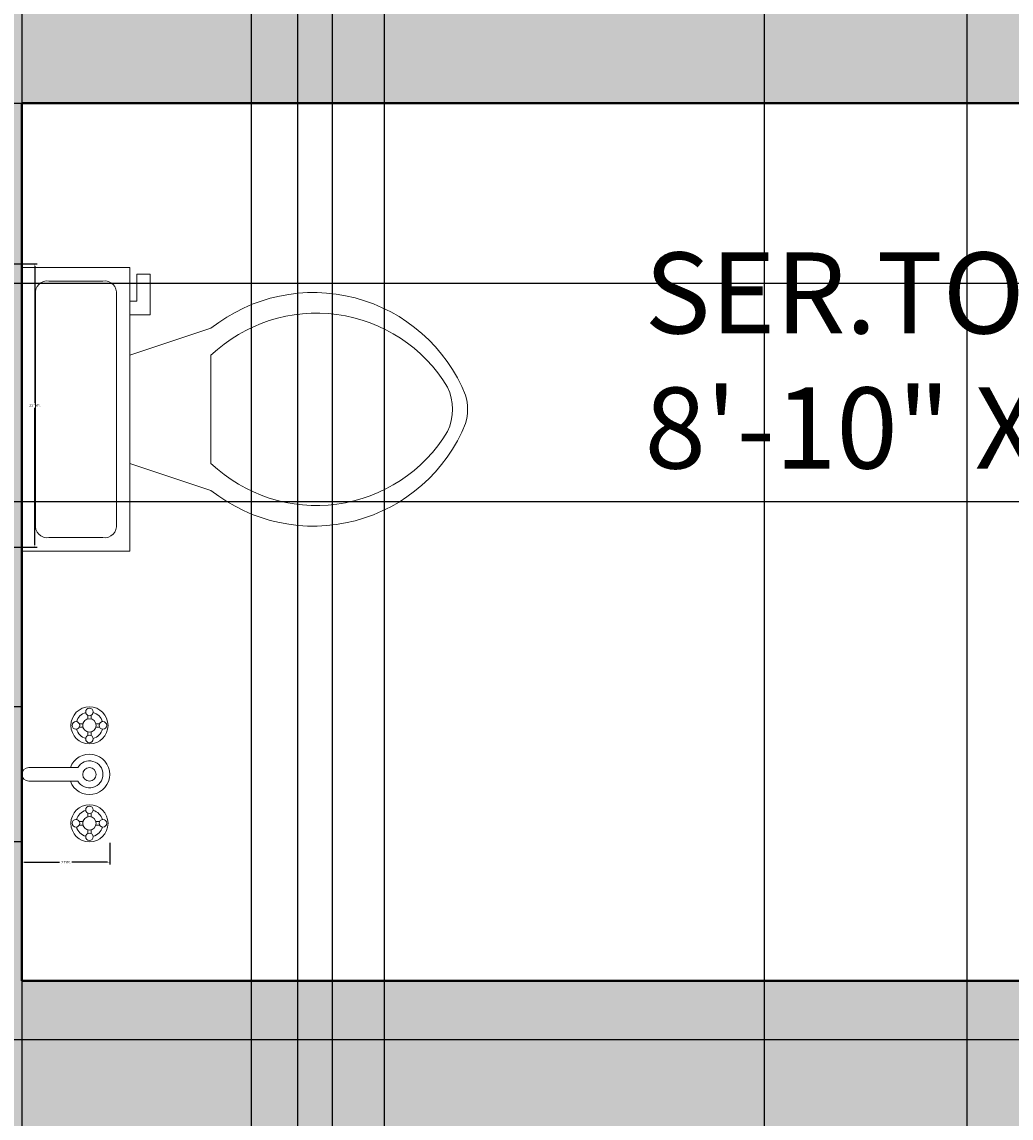
# Model space of a CAD drawing. Units: inches. Extents: x 818 to 1898, y 976 to 2364.
# Tile 54 of 96: x 1600 to 1673, y 1792 to 1873. Entities that reach past the tile are written whole.
import ezdxf

# ---------------------------------------------------------------- set-up
doc = ezdxf.new("R2010")
doc.units = ezdxf.units.IN
doc.header["$LTSCALE"] = 5
doc.header["$MEASUREMENT"] = 0
for name, color, linetype, lineweight in [('A-ANNO-DIMS', 2, 'Continuous', 18), ('A-AREA-IDEN', 7, 'Continuous', 18), ('A-FLOR-FIXT', 9, 'Continuous', 18), ('A-WALL', 7, 'Continuous', 40)]:
    doc.layers.add(name, color=color, linetype=linetype, lineweight=lineweight)
doc.layers.add('A-WALL-PATT', color=251, linetype='Continuous', lineweight=13, true_color=0x636466)
doc.styles.get("Standard").update_dxf_attribs({"font": 'arial.ttf'})
doc.dimstyles.get("Standard").update_dxf_attribs({"dimtxt": 0.18, "dimasz": 0.18, "dimexe": 0.18, "dimexo": 0.0625, "dimgap": 0.09, "dimtad": 0, "dimtih": 1, "dimtoh": 1, "dimdec": 4, "dimzin": 0, "dimdsep": 46, "dimtxsty": 'Standard', "dimcen": 0.09, "dimadec": 0, "dimazin": 0, "dimtfac": 1, "dimtdec": 4, "dimtofl": 0, "dimtmove": 0, "dimatfit": 3, "dimfxl": 1, "dimtolj": 1, "dimtzin": 0, "dimarcsym": 0})

# ---------------------------------------------------------------- blocks, each defined once
blk = doc.blocks.new('Toilet - top')
for p, q in [((9.5, -6), (9.5, -2)), ((-8, -8.5), (-8, -8)), ((-7, -8), (-7, -9.5)), ((-4, -8), (-6, -14)), ((4, -8), (6, -14)), ((-10, -8.5), (-8, -8.5)), ((-10, -9.5), (-10, -8.5)), ((-7, -9.5), (-10, -9.5)), ((4, -14), (-4, -14))]:
    blk.add_line(p, q)
blk.add_lwpolyline([(10.5, -8), (10.5, 0), (-10.5, 0), (-10.5, -8)], close=True)
for points in [[(8.5, -1), (-8.5, -1)], [(-9.5, -2), (-9.5, -6)], [(-8.5, -7), (8.5, -7)]]:
    blk.add_lwpolyline(points)
for centre, radius, start, end in [((-8.625, -1.875), 0.884, 81.8699, 188.1301), ((8.625, -1.875), 0.884, 351.8699, 98.1301), ((-8.625, -6.125), 0.884, 171.8699, 278.1301), ((8.625, -6.125), 0.884, 261.8699, 8.1301), ((3.52, -21.58), 12.169, 141.46911, 247.97143), ((4.2, -21.817), 11.329, 136.36773, 238.94682), ((-3.519, -21.58), 12.169, 292.02843, 38.53071), ((-4.2, -21.817), 11.329, 301.05301, 43.63209), ((0, -27.876), 4, 245.73182, 294.26817), ((0, -29), 4, 254.86053, 285.13947)]:
    blk.add_arc(centre, radius, start, end)
blk = doc.blocks.new('Faucet - Bathroom top')
for p, q in [((-4.107, 0.125), (-4.375, 0.125)), ((-3.75, 0.4788), (-3.75, 0.75)), ((-3.5, 0.482), (-3.5, 0.75)), ((-3.1461, 0.125), (-2.875, 0.125)), ((3.143, 0.125), (2.875, 0.125)), ((3.5, 0.4788), (3.5, 0.75)), ((3.75, 0.482), (3.75, 0.75)), ((4.1039, 0.125), (4.375, 0.125)), ((-4.1039, -0.125), (-4.375, -0.125)), ((-3.75, -0.4821), (-3.75, -0.75)), ((-3.5, -0.4789), (-3.5, -0.75)), ((-3.143, -0.125), (-2.875, -0.125)), ((3.1461, -0.125), (2.875, -0.125)), ((3.5, -0.4821), (3.5, -0.75)), ((3.75, -0.4789), (3.75, -0.75)), ((4.107, -0.125), (4.375, -0.125)), ((-0.5, -0.8639), (-0.5, -4.5)), ((0.5, -4.5), (0.5, -0.8631))]:
    blk.add_line(p, q)
for centre, radius in [((-3.625, 0), 1.375), ((-3.625, 1), 0.2795), ((3.625, 0), 1.375), ((3.625, 1), 0.2795), ((-4.625, 0), 0.2795), ((-3.625, 0), 0.5), ((-2.625, 0), 0.2795), ((0, 0), 0.5), ((2.625, 0), 0.2795), ((3.625, 0), 0.5), ((4.625, 0), 0.2795), ((-3.625, -1), 0.2795), ((3.625, -1), 0.2795)]:
    blk.add_circle(centre, radius)
for centre, radius, start, end in [((-3.625, 0), 1, 105.2407, 164.2093), ((-3.625, 0), 1, 16.44125, 74.07887), ((0, 0), 1.5, 289.6514, 250.3603), ((0, 0), 1, 300.3431, 239.7554), ((3.625, 0), 1, 106.12, 164.0884), ((3.625, 0), 1, 16.23422, 73.90469), ((-3.625, 0), 1, 196.2342, 253.9047), ((-3.625, 0), 1, 286.12, 344.0884), ((3.625, 0), 1, 196.4413, 254.0789), ((3.625, 0), 1, 285.2407, 344.2093), ((0, -4.5), 0.5, 180, 0)]:
    blk.add_arc(centre, radius, start, end)
blk = doc.blocks.new('*D36')
at = {"layer": 'A-ANNO-DIMS', "color": 0, "lineweight": -2, "ltscale": 5, "transparency": 16777216}
for p, q in [((1599.663, 1822.366), (1598.045, 1822.366)), ((1598.225, 1822.186), (1598.225, 1817.548)), ((1598.225, 1812.546), (1598.225, 1817.184)), ((1599.663, 1812.366), (1598.045, 1812.366))]:
    blk.add_line(p, q, dxfattribs=at)
at = {"layer": 'A-ANNO-DIMS', "color": 0, "ltscale": 5, "transparency": 16777216}
for points in [[(1598.195, 1822.186), (1598.255, 1822.186), (1598.225, 1822.366)], [(1598.195, 1812.546), (1598.255, 1812.546), (1598.225, 1812.366)]]:
    blk.add_solid(points, dxfattribs=at)
at = {"layer": 'Defpoints', "color": 0, "ltscale": 5, "transparency": 16777216}
for p in [(1599.725, 1822.366), (1598.225, 1812.366), (1599.725, 1812.366)]:
    blk.add_point(p, dxfattribs=at)
at = {"layer": 'A-ANNO-DIMS', "color": 0, "ltscale": 5, "transparency": 16777216, "insert": (1598.225, 1817.366), "char_height": 0.18, "attachment_point": 5}
blk.add_mtext('\\A1;TAP 10 TYP.', dxfattribs=at)
blk = doc.blocks.new('*D37')
at = {"layer": 'A-ANNO-DIMS', "color": 0, "lineweight": -2, "ltscale": 5, "transparency": 16777216}
for p, q in [((1599.725, 1812.304), (1599.725, 1810.686)), ((1606.225, 1812.304), (1606.225, 1810.686)), ((1599.905, 1810.866), (1602.518, 1810.866)), ((1606.045, 1810.866), (1603.433, 1810.866))]:
    blk.add_line(p, q, dxfattribs=at)
at = {"layer": 'A-ANNO-DIMS', "color": 0, "ltscale": 5, "transparency": 16777216}
for points in [[(1599.905, 1810.896), (1599.905, 1810.836), (1599.725, 1810.866)], [(1606.045, 1810.896), (1606.045, 1810.836), (1606.225, 1810.866)]]:
    blk.add_solid(points, dxfattribs=at)
at = {"layer": 'Defpoints', "color": 0, "ltscale": 5, "transparency": 16777216}
for p in [(1599.725, 1812.366), (1606.225, 1812.366), (1606.225, 1810.866)]:
    blk.add_point(p, dxfattribs=at)
at = {"layer": 'A-ANNO-DIMS', "color": 0, "ltscale": 5, "transparency": 16777216, "insert": (1602.975, 1810.866), "char_height": 0.18, "attachment_point": 5}
blk.add_mtext('\\A1;7 TYP.', dxfattribs=at)
blk = doc.blocks.new('*D41')
at = {"layer": 'A-ANNO-DIMS', "color": 0, "lineweight": -2, "ltscale": 5, "transparency": 16777216}
for p, q in [((1595.788, 1855.184), (1600.862, 1855.184)), ((1600.682, 1855.004), (1600.682, 1844.865)), ((1600.682, 1834.364), (1600.682, 1844.504)), ((1595.788, 1834.184), (1600.862, 1834.184))]:
    blk.add_line(p, q, dxfattribs=at)
at = {"layer": 'A-ANNO-DIMS', "color": 0, "ltscale": 5, "transparency": 16777216}
for points in [[(1600.652, 1855.004), (1600.712, 1855.004), (1600.682, 1855.184)], [(1600.652, 1834.364), (1600.712, 1834.364), (1600.682, 1834.184)]]:
    blk.add_solid(points, dxfattribs=at)
at = {"layer": 'Defpoints', "color": 0, "ltscale": 5, "transparency": 16777216}
for p in [(1595.725, 1855.184), (1595.725, 1834.184), (1600.682, 1834.184)]:
    blk.add_point(p, dxfattribs=at)
at = {"layer": 'A-ANNO-DIMS', "color": 0, "ltscale": 5, "transparency": 16777216, "insert": (1600.682, 1844.684), "char_height": 0.18, "attachment_point": 5}
blk.add_mtext('\\A1;21 TYP.', dxfattribs=at)
blk = doc.blocks.new('*D85')
at = {"layer": 'A-ANNO-DIMS', "color": 0, "lineweight": -2, "ltscale": 5, "transparency": 16777216}
for p, q in [((1258.788, 2053.078), (1897.916, 2053.078)), ((1897.736, 2052.898), (1897.736, 1876.76)), ((1897.736, 1700.258), (1897.736, 1876.396)), ((1258.788, 1700.078), (1897.916, 1700.078))]:
    blk.add_line(p, q, dxfattribs=at)
at = {"layer": 'A-ANNO-DIMS', "color": 0, "ltscale": 5, "transparency": 16777216}
for points in [[(1897.706, 2052.898), (1897.766, 2052.898), (1897.736, 2053.078)], [(1897.706, 1700.258), (1897.766, 1700.258), (1897.736, 1700.078)]]:
    blk.add_solid(points, dxfattribs=at)
at = {"layer": 'Defpoints', "color": 0, "ltscale": 5, "transparency": 16777216}
for p in [(1258.725, 2053.078), (1897.736, 2053.078), (1258.725, 1700.078)]:
    blk.add_point(p, dxfattribs=at)
at = {"layer": 'A-ANNO-DIMS', "color": 0, "ltscale": 5, "transparency": 16777216, "insert": (1897.736, 1876.578), "char_height": 0.18, "attachment_point": 5}
blk.add_mtext('\\A1;353', dxfattribs=at)
blk = doc.blocks.new('*D102')
at = {"layer": 'A-ANNO-DIMS', "color": 0, "lineweight": -2, "ltscale": 5, "transparency": 16777216}
for p, q in [((1565.483, 1071.118), (1565.483, 2363.873)), ((1565.663, 2363.693), (1595.635, 2363.693)), ((1626.395, 2363.693), (1596.423, 2363.693)), ((1626.575, 1071.118), (1626.575, 2363.873))]:
    blk.add_line(p, q, dxfattribs=at)
at = {"layer": 'A-ANNO-DIMS', "color": 0, "ltscale": 5, "transparency": 16777216}
for points in [[(1565.663, 2363.723), (1565.663, 2363.663), (1565.483, 2363.693)], [(1626.395, 2363.723), (1626.395, 2363.663), (1626.575, 2363.693)]]:
    blk.add_solid(points, dxfattribs=at)
at = {"layer": 'Defpoints', "color": 0, "ltscale": 5, "transparency": 16777216}
for p in [(1626.575, 2363.693), (1565.483, 1071.055), (1626.575, 1071.055)]:
    blk.add_point(p, dxfattribs=at)
at = {"layer": 'A-ANNO-DIMS', "color": 0, "ltscale": 5, "transparency": 16777216, "insert": (1596.029, 2363.693), "char_height": 0.18, "attachment_point": 5}
blk.add_mtext('\\A1;61.09', dxfattribs=at)
blk = doc.blocks.new('*D103')
at = {"layer": 'A-ANNO-DIMS', "color": 0, "lineweight": -2, "ltscale": 5, "transparency": 16777216}
for p, q in [((1626.575, 1071.118), (1626.575, 2363.873)), ((1626.755, 2363.693), (1657.699, 2363.693)), ((1689.291, 2363.693), (1658.348, 2363.693)), ((1689.471, 1071.118), (1689.471, 2363.873))]:
    blk.add_line(p, q, dxfattribs=at)
at = {"layer": 'A-ANNO-DIMS', "color": 0, "ltscale": 5, "transparency": 16777216}
for points in [[(1626.755, 2363.723), (1626.755, 2363.663), (1626.575, 2363.693)], [(1689.291, 2363.723), (1689.291, 2363.663), (1689.471, 2363.693)]]:
    blk.add_solid(points, dxfattribs=at)
at = {"layer": 'Defpoints', "color": 0, "ltscale": 5, "transparency": 16777216}
for p in [(1689.471, 2363.693), (1626.575, 1071.055), (1689.471, 1071.055)]:
    blk.add_point(p, dxfattribs=at)
at = {"layer": 'A-ANNO-DIMS', "color": 0, "ltscale": 5, "transparency": 16777216, "insert": (1658.023, 2363.693), "char_height": 0.18, "attachment_point": 5}
blk.add_mtext('\\A1;62.9', dxfattribs=at)
blk = doc.blocks.new('*D120')
at = {"layer": 'A-ANNO-DIMS', "color": 0, "lineweight": -2, "ltscale": 5, "transparency": 16777216}
for p, q in [((1766.29, 1797.717), (818.026, 1797.717)), ((818.206, 1797.537), (818.206, 1757.534)), ((818.206, 1717.167), (818.206, 1757.17)), ((1766.29, 1716.987), (818.026, 1716.987))]:
    blk.add_line(p, q, dxfattribs=at)
at = {"layer": 'A-ANNO-DIMS', "color": 0, "ltscale": 5, "transparency": 16777216}
for points in [[(818.176, 1797.537), (818.236, 1797.537), (818.206, 1797.717)], [(818.176, 1717.167), (818.236, 1717.167), (818.206, 1716.987)]]:
    blk.add_solid(points, dxfattribs=at)
at = {"layer": 'Defpoints', "color": 0, "ltscale": 5, "transparency": 16777216}
for p in [(818.206, 1797.717), (1766.352, 1797.717), (1766.352, 1716.987)]:
    blk.add_point(p, dxfattribs=at)
at = {"layer": 'A-ANNO-DIMS', "color": 0, "ltscale": 5, "transparency": 16777216, "insert": (818.206, 1757.352), "char_height": 0.18, "attachment_point": 5}
blk.add_mtext('\\A1;80.73', dxfattribs=at)
blk = doc.blocks.new('*D121')
at = {"layer": 'A-ANNO-DIMS', "color": 0, "lineweight": -2, "ltscale": 5, "transparency": 16777216}
for p, q in [((1766.29, 1884.203), (818.026, 1884.203)), ((818.206, 1884.023), (818.206, 1841.142)), ((818.206, 1797.897), (818.206, 1840.778)), ((1766.29, 1797.717), (818.026, 1797.717))]:
    blk.add_line(p, q, dxfattribs=at)
at = {"layer": 'A-ANNO-DIMS', "color": 0, "ltscale": 5, "transparency": 16777216}
for points in [[(818.176, 1884.023), (818.236, 1884.023), (818.206, 1884.203)], [(818.176, 1797.897), (818.236, 1797.897), (818.206, 1797.717)]]:
    blk.add_solid(points, dxfattribs=at)
at = {"layer": 'Defpoints', "color": 0, "ltscale": 5, "transparency": 16777216}
for p in [(818.206, 1884.203), (1766.352, 1884.203), (1766.352, 1797.717)]:
    blk.add_point(p, dxfattribs=at)
at = {"layer": 'A-ANNO-DIMS', "color": 0, "ltscale": 5, "transparency": 16777216, "insert": (818.206, 1840.96), "char_height": 0.18, "attachment_point": 5}
blk.add_mtext('\\A1;86.49', dxfattribs=at)
blk = doc.blocks.new('*D173')
at = {"layer": 'A-ANNO-DIMS', "color": 0, "lineweight": -2, "ltscale": 5, "transparency": 16777216}
for p, q in [((1622.725, 1463.141), (1622.725, 2363.873)), ((1622.905, 2363.693), (1638.507, 2363.693)), ((1654.545, 2363.693), (1638.943, 2363.693)), ((1654.725, 1463.141), (1654.725, 2363.873))]:
    blk.add_line(p, q, dxfattribs=at)
at = {"layer": 'A-ANNO-DIMS', "color": 0, "ltscale": 5, "transparency": 16777216}
for points in [[(1622.905, 2363.723), (1622.905, 2363.663), (1622.725, 2363.693)], [(1654.545, 2363.723), (1654.545, 2363.663), (1654.725, 2363.693)]]:
    blk.add_solid(points, dxfattribs=at)
at = {"layer": 'Defpoints', "color": 0, "ltscale": 5, "transparency": 16777216}
for p in [(1654.725, 2363.693), (1622.725, 1463.078), (1654.725, 1463.078)]:
    blk.add_point(p, dxfattribs=at)
at = {"layer": 'A-ANNO-DIMS', "color": 0, "ltscale": 5, "transparency": 16777216, "insert": (1638.725, 2363.693), "char_height": 0.18, "attachment_point": 5}
blk.add_mtext('\\A1;32', dxfattribs=at)
blk = doc.blocks.new('*D174')
at = {"layer": 'A-ANNO-DIMS', "color": 0, "lineweight": -2, "ltscale": 5, "transparency": 16777216}
for p, q in [((1616.725, 1416.748), (1616.725, 2363.873)), ((1616.905, 2363.693), (1619.576, 2363.693)), ((1622.545, 2363.693), (1619.875, 2363.693)), ((1622.725, 1416.748), (1622.725, 2363.873))]:
    blk.add_line(p, q, dxfattribs=at)
at = {"layer": 'A-ANNO-DIMS', "color": 0, "ltscale": 5, "transparency": 16777216}
for points in [[(1616.905, 2363.723), (1616.905, 2363.663), (1616.725, 2363.693)], [(1622.545, 2363.723), (1622.545, 2363.663), (1622.725, 2363.693)]]:
    blk.add_solid(points, dxfattribs=at)
at = {"layer": 'Defpoints', "color": 0, "ltscale": 5, "transparency": 16777216}
for p in [(1622.725, 2363.693), (1616.725, 1416.686), (1622.725, 1416.686)]:
    blk.add_point(p, dxfattribs=at)
at = {"layer": 'A-ANNO-DIMS', "color": 0, "ltscale": 5, "transparency": 16777216, "insert": (1619.725, 2363.693), "char_height": 0.18, "attachment_point": 5}
blk.add_mtext('\\A1;6', dxfattribs=at)
blk = doc.blocks.new('*D175')
at = {"layer": 'A-ANNO-DIMS', "color": 0, "lineweight": -2, "ltscale": 5, "transparency": 16777216}
for p, q in [((1559.725, 1647.641), (1559.725, 2363.873)), ((1559.905, 2363.693), (1614.445, 2363.693)), ((1669.545, 2363.693), (1615.005, 2363.693)), ((1669.725, 1647.641), (1669.725, 2363.873))]:
    blk.add_line(p, q, dxfattribs=at)
at = {"layer": 'A-ANNO-DIMS', "color": 0, "ltscale": 5, "transparency": 16777216}
for points in [[(1559.905, 2363.723), (1559.905, 2363.663), (1559.725, 2363.693)], [(1669.545, 2363.723), (1669.545, 2363.663), (1669.725, 2363.693)]]:
    blk.add_solid(points, dxfattribs=at)
at = {"layer": 'Defpoints', "color": 0, "ltscale": 5, "transparency": 16777216}
for p in [(1669.725, 2363.693), (1559.725, 1647.578), (1669.725, 1647.578)]:
    blk.add_point(p, dxfattribs=at)
at = {"layer": 'A-ANNO-DIMS', "color": 0, "ltscale": 5, "transparency": 16777216, "insert": (1614.725, 2363.693), "char_height": 0.18, "attachment_point": 5}
blk.add_mtext('\\A1;110', dxfattribs=at)
blk = doc.blocks.new('*D225')
at = {"layer": 'A-ANNO-DIMS', "color": 0, "lineweight": -2, "ltscale": 5, "transparency": 16777216}
for p, q in [((1532.655, 1867.078), (1897.916, 1867.078)), ((1897.736, 1866.898), (1897.736, 1852.512)), ((1897.736, 1837.762), (1897.736, 1852.148)), ((1532.655, 1837.582), (1897.916, 1837.582))]:
    blk.add_line(p, q, dxfattribs=at)
at = {"layer": 'A-ANNO-DIMS', "color": 0, "ltscale": 5, "transparency": 16777216}
for points in [[(1897.706, 1866.898), (1897.766, 1866.898), (1897.736, 1867.078)], [(1897.706, 1837.762), (1897.766, 1837.762), (1897.736, 1837.582)]]:
    blk.add_solid(points, dxfattribs=at)
at = {"layer": 'Defpoints', "color": 0, "ltscale": 5, "transparency": 16777216}
for p in [(1532.593, 1867.078), (1897.736, 1867.078), (1532.593, 1837.582)]:
    blk.add_point(p, dxfattribs=at)
at = {"layer": 'A-ANNO-DIMS', "color": 0, "ltscale": 5, "transparency": 16777216, "insert": (1897.736, 1852.33), "char_height": 0.18, "attachment_point": 5}
blk.add_mtext('\\A1;29.496', dxfattribs=at)
blk = doc.blocks.new('*D229')
at = {"layer": 'A-ANNO-DIMS', "color": 0, "lineweight": -2, "ltscale": 5, "transparency": 16777216}
for p, q in [((1599.725, 2044.016), (1599.725, 975.663)), ((1620.142, 2036.056), (1620.142, 975.663)), ((1599.905, 975.843), (1609.468, 975.843)), ((1619.962, 975.843), (1610.398, 975.843))]:
    blk.add_line(p, q, dxfattribs=at)
at = {"layer": 'A-ANNO-DIMS', "color": 0, "ltscale": 5, "transparency": 16777216}
for points in [[(1599.905, 975.873), (1599.905, 975.813), (1599.725, 975.843)], [(1619.962, 975.873), (1619.962, 975.813), (1620.142, 975.843)]]:
    blk.add_solid(points, dxfattribs=at)
at = {"layer": 'Defpoints', "color": 0, "ltscale": 5, "transparency": 16777216}
for p in [(1599.725, 2044.078), (1620.142, 2036.118), (1620.142, 975.843)]:
    blk.add_point(p, dxfattribs=at)
at = {"layer": 'A-ANNO-DIMS', "color": 0, "ltscale": 5, "transparency": 16777216, "insert": (1609.933, 975.843), "char_height": 0.18, "attachment_point": 5}
blk.add_mtext('\\A1;20.416', dxfattribs=at)
blk = doc.blocks.new('*D275')
at = {"layer": 'A-ANNO-DIMS', "color": 0, "lineweight": -2, "ltscale": 5, "transparency": 16777216}
for p, q in [((1377.842, 1897.866), (1897.916, 1897.866)), ((1897.736, 1897.686), (1897.736, 1875.988)), ((1897.736, 1853.93), (1897.736, 1875.628)), ((1377.842, 1853.75), (1897.916, 1853.75))]:
    blk.add_line(p, q, dxfattribs=at)
at = {"layer": 'A-ANNO-DIMS', "color": 0, "ltscale": 5, "transparency": 16777216}
for points in [[(1897.706, 1897.686), (1897.766, 1897.686), (1897.736, 1897.866)], [(1897.706, 1853.93), (1897.766, 1853.93), (1897.736, 1853.75)]]:
    blk.add_solid(points, dxfattribs=at)
at = {"layer": 'Defpoints', "color": 0, "ltscale": 5, "transparency": 16777216}
for p in [(1377.779, 1897.866), (1897.736, 1897.866), (1377.779, 1853.75)]:
    blk.add_point(p, dxfattribs=at)
at = {"layer": 'A-ANNO-DIMS', "color": 0, "ltscale": 5, "transparency": 16777216, "insert": (1897.736, 1875.808), "char_height": 0.18, "attachment_point": 5}
blk.add_mtext('\\A1;44.12', dxfattribs=at)
blk = doc.blocks.new('*D282')
at = {"layer": 'A-ANNO-DIMS', "color": 0, "lineweight": -2, "ltscale": 5, "transparency": 16777216}
for p, q in [((1422.083, 2081.188), (1897.916, 2081.188)), ((1897.736, 2081.008), (1897.736, 1884.315)), ((1897.736, 1687.258), (1897.736, 1883.951)), ((1463.788, 1687.078), (1897.916, 1687.078))]:
    blk.add_line(p, q, dxfattribs=at)
at = {"layer": 'A-ANNO-DIMS', "color": 0, "ltscale": 5, "transparency": 16777216}
for points in [[(1897.706, 2081.008), (1897.766, 2081.008), (1897.736, 2081.188)], [(1897.706, 1687.258), (1897.766, 1687.258), (1897.736, 1687.078)]]:
    blk.add_solid(points, dxfattribs=at)
at = {"layer": 'Defpoints', "color": 0, "ltscale": 5, "transparency": 16777216}
for p in [(1422.02, 2081.188), (1897.736, 2081.188), (1463.725, 1687.078)]:
    blk.add_point(p, dxfattribs=at)
at = {"layer": 'A-ANNO-DIMS', "color": 0, "ltscale": 5, "transparency": 16777216, "insert": (1897.736, 1884.133), "char_height": 0.18, "attachment_point": 5}
blk.add_mtext('\\A1;394.1', dxfattribs=at)

msp = doc.modelspace()

# ---------------------------------------------------------------- hatches: boundary and pattern name
at = {"layer": 'A-WALL-PATT', "ltscale": 5}
h = msp.add_hatch(color=256, dxfattribs=at)
h.dxf.hatch_style = 1
h.paths.add_polyline_path([(1267.7252, 1928.9218), (1258.7251, 1928.9218), (1258.7251, 1913.6401), (1250.3029, 1913.6401), (1250.3029, 1878.3919), (1258.7251, 1878.3919), (1258.7251, 1862.9652), (1267.7252, 1862.9652)])
h.paths.add_polyline_path([(1267.7252, 1814.9652), (1258.7251, 1814.9652), (1258.7251, 1755.3321), (1267.7252, 1755.3321)])
h.paths.add_polyline_path([(1463.7251, 1696.0782), (1267.7252, 1696.0782), (1267.7252, 1707.3321), (1258.7251, 1707.3321), (1258.7251, 1700.0782), (1251.9333, 1700.0782), (1251.9333, 1687.0782), (1463.7251, 1687.0782)])
h.paths.add_polyline_path([(1714.7252, 1717.3178), (1705.7252, 1717.3178), (1705.7252, 1696.0782), (1599.7251, 1696.0782), (1599.7251, 1790.0782), (1705.7252, 1790.0782), (1705.7252, 1785.6125), (1714.7252, 1785.6125), (1714.7252, 1827.2125), (1705.7252, 1827.2125), (1705.7252, 1802.0782), (1599.7251, 1802.0782), (1599.7251, 1867.0782), (1705.7252, 1867.0782), (1705.7252, 1857.2125), (1714.7252, 1857.2125), (1714.7252, 1930.0316), (1741.8409, 1930.0316), (1741.8409, 1935.0316), (1714.7252, 1935.0316), (1714.7252, 1957.0338), (1741.8409, 1957.0338), (1741.8409, 1962.0338), (1714.7252, 1962.0338), (1705.7252, 1962.0338), (1705.7252, 1948.0782), (1599.7251, 1948.0782), (1599.7251, 1981.0782), (1590.7252, 1981.0782), (1590.7252, 1941.0782), (1620.7252, 1941.0782), (1705.7252, 1941.0782), (1705.7252, 1876.0782), (1599.7251, 1876.0782), (1599.7251, 1911.0782), (1590.7252, 1911.0782), (1590.7252, 1876.0782), (1429.2252, 1876.0782), (1429.2252, 1867.0782), (1511.7252, 1867.0782), (1528.593, 1867.0782), (1595.7252, 1867.0782), (1595.7252, 1773.0782), (1520.7252, 1773.0782), (1520.7252, 1837.5823), (1532.593, 1837.5823), (1532.593, 1867.0782), (1528.593, 1867.0782), (1528.593, 1841.5823), (1511.7252, 1841.5823), (1511.7252, 1744.9714), (1520.7252, 1744.9714), (1520.7252, 1761.0782), (1595.7252, 1761.0782), (1595.7252, 1696.0782), (1520.7252, 1696.0782), (1520.7252, 1716.0454), (1511.7252, 1716.0454), (1511.7252, 1696.0782), (1511.7252, 1687.0782), (1714.7252, 1687.0782)])
h.paths.add_polyline_path([(1714.7252, 2053.0782), (1714.7252, 2081.1881), (1709.7252, 2081.1881), (1709.7252, 2053.0782), (1681.6446, 2053.0782), (1681.6446, 2081.1881), (1676.6446, 2081.1881), (1676.6446, 2053.0782), (1538.5155, 2053.0782), (1538.5155, 2044.0782), (1590.7252, 2044.0782), (1590.7252, 2011.0782), (1599.7251, 2011.0782), (1599.7251, 2044.0782), (1705.7252, 2044.0782), (1705.7252, 2014.5114), (1714.7252, 2014.5114)])
h.paths.add_polyline_path([(1485.1216, 2053.0782), (1422.02, 2053.0782), (1422.02, 2081.1881), (1413.02, 2081.1881), (1413.02, 2053.0782), (1399.6356, 2053.0782), (1399.6356, 2081.1881), (1390.6356, 2081.1881), (1390.6356, 2053.0782), (1388.0315, 2053.0782), (1388.0315, 2044.0782), (1416.2743, 2044.0782), (1485.1216, 2044.0782)])
h.paths.add_polyline_path([(1330.305, 2053.0782), (1258.7251, 2053.0782), (1258.7251, 2019.2871), (1267.7252, 2019.2871), (1267.7252, 2044.0782), (1330.305, 2044.0782)])
h.paths.add_polyline_path([(1258.7251, 2053.0782), (1214.6577, 2053.0782), (1214.6577, 2044.0782), (1258.7251, 2044.0782)])
h.paths.add_polyline_path([(1214.6577, 2053.0782), (1180.349, 2053.0782), (1180.349, 2044.0782), (1214.6577, 2044.0782)])
h.paths.add_polyline_path([(1714.7252, 1639.5782), (1741.8409, 1639.5782), (1741.8409, 1643.5782), (1714.7252, 1643.5782), (1714.7252, 1649.9029), (1705.7252, 1649.9029), (1705.7252, 1600.0782), (1477.7252, 1600.0782), (1477.7252, 1591.0782), (1520.7252, 1591.0782), (1616.7251, 1591.0782), (1616.7251, 1416.6857), (1622.7251, 1416.6857), (1622.7251, 1463.0782), (1624.7252, 1463.0782), (1624.7252, 1467.0782), (1622.7251, 1467.0782), (1622.7251, 1591.0782), (1705.7252, 1591.0782), (1705.7252, 1545.0782), (1714.7252, 1545.0782), (1741.8409, 1545.0782), (1741.8409, 1549.0782), (1714.7252, 1549.0782), (1714.7252, 1593.9175), (1737.8409, 1593.9175), (1737.8409, 1597.9175), (1714.7252, 1597.9175)])
h.paths.add_polyline_path([(1674.9024, 2060.7419), (1714.7045, 2060.7419), (1714.7045, 2073.1061), (1674.9024, 2073.1061)], flags=25)
h.paths.add_polyline_path([(1394.5468, 2061.6618), (1422.2344, 2061.6618), (1422.2344, 2074.0261), (1394.5468, 2074.0261)], flags=24)

# ---------------------------------------------------------------- linework, layer by layer
at = {"layer": 'A-WALL'}
for p, q in [((1599.7251, 1867.0782), (1705.7252, 1867.0782)), ((1599.7251, 1867.0782), (1599.7251, 1802.0782)), ((1599.7251, 1802.0782), (1705.7252, 1802.0782))]:
    msp.add_line(p, q, dxfattribs=at)

# ---------------------------------------------------------------- block references
at = {"layer": 'A-FLOR-FIXT', "xscale": -1, "rotation": 90}
msp.add_blockref('Toilet - top', (1599.7251, 1844.4024), dxfattribs=at)
at = {"layer": 'A-FLOR-FIXT', "rotation": 270}
msp.add_blockref('Faucet - Bathroom top', (1604.7252, 1817.3662), dxfattribs=at)

# ---------------------------------------------------------------- texts
at = {"layer": 'A-AREA-IDEN', "ltscale": 5, "insert": (1645.8362, 1856.0216), "char_height": 6, "attachment_point": 1}
msp.add_mtext_dynamic_manual_height_columns('SER.TOILET\\P8\'-10" X 5\'-5"', width=118.992422, gutter_width=1, heights=[0], dxfattribs=at)

# ---------------------------------------------------------------- dimensions: what is measured, and where the dimension line sits
at = {"layer": 'A-ANNO-DIMS', "ltscale": 5}
for base, p1, p2, override, picture, middle in [((1669.7251, 2363.6929), (1559.7251, 1647.5782), (1669.7251, 1647.5782), {"dimdec": 0, "dimlfac": 1, "dimrnd": 0, "dimzin": 0, "dimdsep": 46, "dimlunit": 2}, '*D175', (1614.7251, 2363.6929)), ((1626.5748, 2363.6929), (1565.4835, 1071.0552), (1626.5748, 1071.0552), {"dimdec": 2, "dimlfac": 1, "dimrnd": 0, "dimzin": 0, "dimdsep": 46, "dimlunit": 2}, '*D102', (1596.0291, 2363.6929)), ((1622.7251, 2363.6929), (1616.7251, 1416.6857), (1622.7251, 1416.6857), {"dimdec": 0, "dimlfac": 1, "dimrnd": 0, "dimzin": 0, "dimdsep": 46, "dimlunit": 2}, '*D174', (1619.7251, 2363.6929)), ((1654.7251, 2363.6929), (1622.7251, 1463.0782), (1654.7251, 1463.0782), {"dimdec": 0, "dimlfac": 1, "dimrnd": 0, "dimzin": 0, "dimdsep": 46, "dimlunit": 2}, '*D173', (1638.7251, 2363.6929)), ((1689.4714, 2363.6929), (1626.5748, 1071.0552), (1689.4714, 1071.0552), {"dimdec": 1, "dimlfac": 1, "dimrnd": 0, "dimzin": 0, "dimdsep": 46, "dimlunit": 2}, '*D103', (1658.0231, 2363.6929)), ((1620.14159, 975.84326), (1599.72515, 2044.07824), (1620.14159, 2036.1182), {"dimdec": 3, "dimlfac": 1, "dimrnd": 0, "dimzin": 0, "dimdsep": 46, "dimlunit": 2}, '*D229', (1609.93337, 975.84326))]:
    dim = msp.add_linear_dim(base=base, p1=p1, p2=p2, dimstyle='Standard', override=override, dxfattribs=at)
    dim.commit()
    dim.dimension.update_dxf_attribs({"geometry": picture, "text_midpoint": middle})
for base, p1, p2, override, picture, middle in [((1897.736, 2081.1881), (1463.7251, 1687.0782), (1422.02, 2081.1881), {"dimdec": 1, "dimlfac": 1, "dimrnd": 0, "dimzin": 0, "dimdsep": 46, "dimlunit": 2}, '*D282', (1897.736, 1884.1332)), ((1897.736, 2053.0782), (1258.7251, 1700.0782), (1258.7251, 2053.0782), {"dimdec": 0, "dimlfac": 1, "dimrnd": 0, "dimzin": 0, "dimdsep": 46, "dimlunit": 2}, '*D85', (1897.736, 1876.5782)), ((1897.736, 1897.8663), (1377.7791, 1853.7496), (1377.7791, 1897.8663), {"dimdec": 2, "dimlfac": 1, "dimrnd": 0, "dimzin": 0, "dimdsep": 46, "dimlunit": 2}, '*D275', (1897.736, 1875.808)), ((818.2059, 1884.2031), (1766.3524, 1797.7165), (1766.3524, 1884.2031), {"dimdec": 2, "dimlfac": 1, "dimrnd": 0, "dimzin": 0, "dimdsep": 46, "dimlunit": 2}, '*D121', (818.2059, 1840.9598)), ((1897.736, 1867.0782), (1532.593, 1837.5823), (1532.593, 1867.0782), {"dimdec": 3, "dimlfac": 1, "dimrnd": 0, "dimzin": 0, "dimdsep": 46, "dimlunit": 2}, '*D225', (1897.736, 1852.3303)), ((818.2059, 1797.7165), (1766.3524, 1716.9866), (1766.3524, 1797.7165), {"dimdec": 2, "dimlfac": 1, "dimrnd": 0, "dimzin": 0, "dimdsep": 46, "dimlunit": 2}, '*D120', (818.2059, 1757.3516))]:
    dim = msp.add_linear_dim(base=base, p1=p1, p2=p2, angle=90, dimstyle='Standard', override=override, dxfattribs=at)
    dim.commit()
    dim.dimension.update_dxf_attribs({"geometry": picture, "text_midpoint": middle})
for base, p1, p2, text, picture, middle in [((1600.6821, 1834.1844), (1595.7252, 1855.1844), (1595.7252, 1834.1844), '<> TYP.', '*D41', (1600.6821, 1844.6844)), ((1598.2252, 1812.3662), (1599.7251, 1822.3662), (1599.7251, 1812.3662), 'TAP <> TYP.', '*D36', (1598.2252, 1817.3662))]:
    dim = msp.add_linear_dim(base=base, p1=p1, p2=p2, angle=270, text=text, dimstyle='Standard', override={"dimdec": 0, "dimlfac": 1, "dimrnd": 0, "dimzin": 0, "dimdsep": 46, "dimlunit": 2}, dxfattribs=at)
    dim.commit()
    dim.dimension.update_dxf_attribs({"geometry": picture, "text_midpoint": middle})
dim = msp.add_linear_dim(base=(1606.22522, 1810.86623), p1=(1599.72515, 1812.36623), p2=(1606.22522, 1812.36623), text='<> TYP.', dimstyle='Standard', override={"dimdec": 0, "dimlfac": 1, "dimrnd": 0, "dimzin": 0, "dimdsep": 46, "dimlunit": 2}, dxfattribs=at)
dim.commit()
dim.dimension.update_dxf_attribs({"geometry": '*D37', "text_midpoint": (1602.97519, 1810.86623)})

doc.saveas('drawing.dxf')
